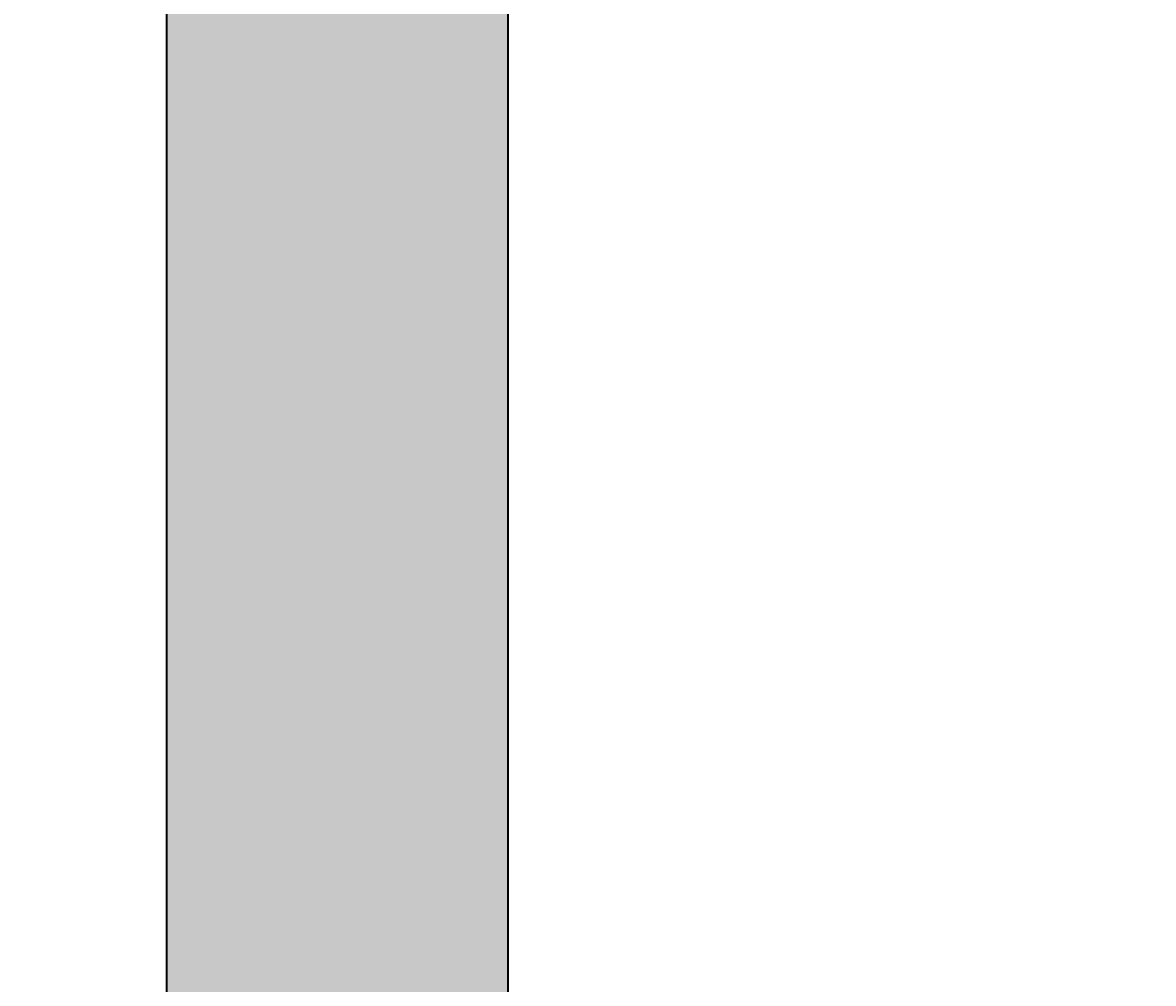
# Model space of a CAD drawing. Units: inches. Extents: x 1998 to 2588, y 1139 to 1977.
# Tile 109 of 134: x 2498 to 2528, y 1427 to 1452. Entities that reach past the tile are written whole.
import ezdxf

# ---------------------------------------------------------------- set-up
doc = ezdxf.new("R2010")
doc.units = ezdxf.units.IN
for name, color, linetype, lineweight in [('A-ANNO-DIMS', 2, 'Continuous', 18), ('A-WALL-PATT', 252, 'Continuous', 13), ('WALL', 200, 'Continuous', 35)]:
    doc.layers.add(name, color=color, linetype=linetype, lineweight=lineweight)
doc.styles.get("Standard").update_dxf_attribs({"font": 'arial.ttf'})
doc.dimstyles.get("Standard").update_dxf_attribs({"dimtxt": 0.18, "dimasz": 0.18, "dimexe": 0.18, "dimexo": 0.0625, "dimgap": 0.09, "dimtad": 0, "dimtih": 1, "dimtoh": 1, "dimdec": 4, "dimzin": 0, "dimdsep": 46, "dimtxsty": 'Standard', "dimcen": 0.09, "dimadec": 0, "dimazin": 0, "dimtfac": 1, "dimtdec": 4, "dimtofl": 0, "dimtmove": 0, "dimatfit": 3, "dimfxl": 1, "dimtolj": 1, "dimtzin": 0, "dimarcsym": 0})

# ---------------------------------------------------------------- blocks, each defined once
blk = doc.blocks.new('*D23')
at = {"layer": 'A-ANNO-DIMS', "color": 0, "lineweight": -2, "transparency": 16777216}
for p, q in [((2549.179, 1476.17), (2549.179, 1138.602)), ((2059.473, 1413.17), (2059.473, 1138.602)), ((2059.653, 1138.782), (2303.928, 1138.782)), ((2548.999, 1138.782), (2304.723, 1138.782))]:
    blk.add_line(p, q, dxfattribs=at)
at = {"layer": 'A-ANNO-DIMS', "color": 0, "transparency": 16777216}
for points in [[(2059.653, 1138.812), (2059.653, 1138.752), (2059.473, 1138.782)], [(2548.999, 1138.812), (2548.999, 1138.752), (2549.179, 1138.782)]]:
    blk.add_solid(points, dxfattribs=at)
at = {"layer": 'Defpoints', "color": 0, "transparency": 16777216}
for p in [(2549.179, 1476.232), (2059.473, 1413.232), (2549.179, 1138.782)]:
    blk.add_point(p, dxfattribs=at)
at = {"layer": 'A-ANNO-DIMS', "color": 0, "transparency": 16777216, "insert": (2304.326, 1138.782), "char_height": 0.18, "attachment_point": 5}
blk.add_mtext('\\A1;489.7', dxfattribs=at)
blk = doc.blocks.new('*D24')
at = {"layer": 'A-ANNO-DIMS', "color": 0, "lineweight": -2, "transparency": 16777216}
for p, q in [((2398.535, 1911.232), (2588.309, 1911.232)), ((2588.129, 1911.052), (2588.129, 1570.164)), ((2588.129, 1228.912), (2588.129, 1569.8)), ((2527.535, 1228.732), (2588.309, 1228.732))]:
    blk.add_line(p, q, dxfattribs=at)
at = {"layer": 'A-ANNO-DIMS', "color": 0, "transparency": 16777216}
for points in [[(2588.099, 1911.052), (2588.159, 1911.052), (2588.129, 1911.232)], [(2588.099, 1228.912), (2588.159, 1228.912), (2588.129, 1228.732)]]:
    blk.add_solid(points, dxfattribs=at)
at = {"layer": 'Defpoints', "color": 0, "transparency": 16777216}
for p in [(2398.473, 1911.232), (2588.129, 1911.232), (2527.473, 1228.732)]:
    blk.add_point(p, dxfattribs=at)
at = {"layer": 'A-ANNO-DIMS', "color": 0, "transparency": 16777216, "insert": (2588.129, 1569.982), "char_height": 0.18, "attachment_point": 5}
blk.add_mtext('\\A1;682.5', dxfattribs=at)

msp = doc.modelspace()

# ---------------------------------------------------------------- hatches: boundary and pattern name
at = {"layer": 'A-WALL-PATT'}
h = msp.add_hatch(color=256, dxfattribs=at)
h.dxf.hatch_style = 1
h.paths.add_polyline_path([(2227.4729, 1911.2324), (2222.9729, 1911.2324), (2222.9729, 1888.7324), (2227.4729, 1888.7324)])
h.paths.add_polyline_path([(2236.4493, 1870.3636), (2236.4493, 1875.2324), (2234.4125, 1875.2324), (2234.4125, 1868.3278), (2227.4729, 1868.3278), (2227.4729, 1866.2324), (2236.4493, 1866.2324)])
h.paths.add_polyline_path([(2330.0332, 1875.2324), (2263.9907, 1875.2324), (2263.9907, 1866.2324), (2330.0332, 1866.2324)])
h.paths.add_polyline_path([(2345.9729, 1906.7324), (2393.9729, 1906.7324), (2393.9729, 1882.7324), (2345.9729, 1882.7324), (2345.9729, 1878.2324), (2393.9729, 1878.2324), (2398.4729, 1878.2324), (2398.4729, 1882.7324), (2398.4729, 1911.2324), (2345.9729, 1911.2324), (2341.4729, 1911.2324), (2341.4729, 1866.2324), (2341.4729, 1790.0412), (2345.9729, 1790.0412), (2345.9729, 1875.2324)])
h.paths.add_polyline_path([(2398.4729, 1878.2324), (2393.9729, 1878.2324), (2393.9729, 1798.2324), (2393.9729, 1793.7324), (2398.4729, 1793.7324)], flags=17)
h.paths.add_polyline_path([(2393.9729, 1798.2324), (2375.7311, 1798.2324, -0.005968), (2375.7384, 1797.6146), (2375.7384, 1793.7324), (2393.9729, 1793.7324)], flags=17)
h.paths.add_polyline_path([(2349.8569, 1797.6146), (2349.8569, 1798.2324), (2345.9729, 1798.2324), (2345.9729, 1793.7324), (2349.8569, 1793.7324)], flags=17)
h.paths.add_polyline_path([(2398.4729, 1793.7324), (2393.9729, 1793.7324), (2393.9729, 1790.0412), (2398.4729, 1790.0412)], flags=17)
h.paths.add_polyline_path([(2527.4729, 1882.7324), (2507.8006, 1882.7324), (2507.8006, 1878.2324), (2518.4729, 1878.2324), (2518.4729, 1759.7324), (2510.9729, 1759.7324), (2510.9729, 1755.2324), (2527.4729, 1755.2324)])
h.paths.add_polyline_path([(2487.396, 1882.7324), (2398.4729, 1882.7324), (2398.4729, 1878.2324), (2487.396, 1878.2324)])
h.paths.add_polyline_path([(2490.5682, 1759.7324), (2345.9729, 1759.7324), (2345.9729, 1755.2324), (2490.5682, 1755.2324)])
h.paths.add_polyline_path([(2398.4729, 1760.5844), (2398.3914, 1760.5844), (2393.9729, 1760.5844), (2393.9729, 1759.7324), (2398.4729, 1759.7324)])
h.paths.add_polyline_path([(2334.5332, 1759.7324), (2234.4125, 1759.7324), (2234.4125, 1755.2324), (2334.5332, 1755.2324)])
h.paths.add_polyline_path([(2345.9729, 1760.5844), (2341.5543, 1760.5844), (2341.4729, 1760.5844), (2341.4729, 1759.7324), (2345.9729, 1759.7324)])
h.paths.add_polyline_path([(2222.9729, 1759.7324), (2221.7204, 1759.7324), (2221.7204, 1755.2324), (2222.9729, 1755.2324)])
h.paths.add_polyline_path([(2061.4729, 1702.7324), (2059.4729, 1702.7324), (2059.4729, 1584.2324), (2061.4729, 1584.2324)])
h.paths.add_polyline_path([(2061.4729, 1584.2324), (2059.4729, 1584.2324), (2059.4729, 1470.2324), (2061.4729, 1470.2324)])
h.paths.add_polyline_path([(2510.9729, 1469.2927), (2501.9729, 1469.2927), (2501.9729, 1369.172), (2510.9729, 1369.172)])
h.paths.add_polyline_path([(2227.4729, 1369.7324), (2227.4729, 1417.7324), (2221.4126, 1417.7324), (2221.4126, 1413.2324), (2222.9729, 1413.2324), (2222.9729, 1293.2324), (2222.9729, 1285.137), (2227.4729, 1285.137)])

# ---------------------------------------------------------------- linework, layer by layer
at = {"layer": 'WALL'}
for p, q in [((2501.9729, 1476.2324), (2501.9729, 1369.172)), ((2510.9729, 1469.2927), (2510.9729, 1357.7324))]:
    msp.add_line(p, q, dxfattribs=at)

# ---------------------------------------------------------------- dimensions: what is measured, and where the dimension line sits
at = {"layer": 'A-ANNO-DIMS'}
dim = msp.add_linear_dim(base=(2588.1286, 1911.2324), p1=(2527.4729, 1228.7324), p2=(2398.4729, 1911.2324), angle=90, dimstyle='Standard', override={"dimdec": 1, "dimlfac": 1, "dimrnd": 0, "dimzin": 0, "dimdsep": 46, "dimlunit": 2}, dxfattribs=at)
dim.commit()
dim.dimension.update_dxf_attribs({"geometry": '*D24', "text_midpoint": (2588.1286, 1569.9824)})
dim = msp.add_linear_dim(base=(2549.1786, 1138.7824), p1=(2059.4729, 1413.2324), p2=(2549.1786, 1476.2324), dimstyle='Standard', override={"dimdec": 1, "dimlfac": 1, "dimrnd": 0, "dimzin": 0, "dimdsep": 46, "dimlunit": 2}, dxfattribs=at)
dim.commit()
dim.dimension.update_dxf_attribs({"geometry": '*D23', "text_midpoint": (2304.3257, 1138.7824)})

doc.saveas('drawing.dxf')
